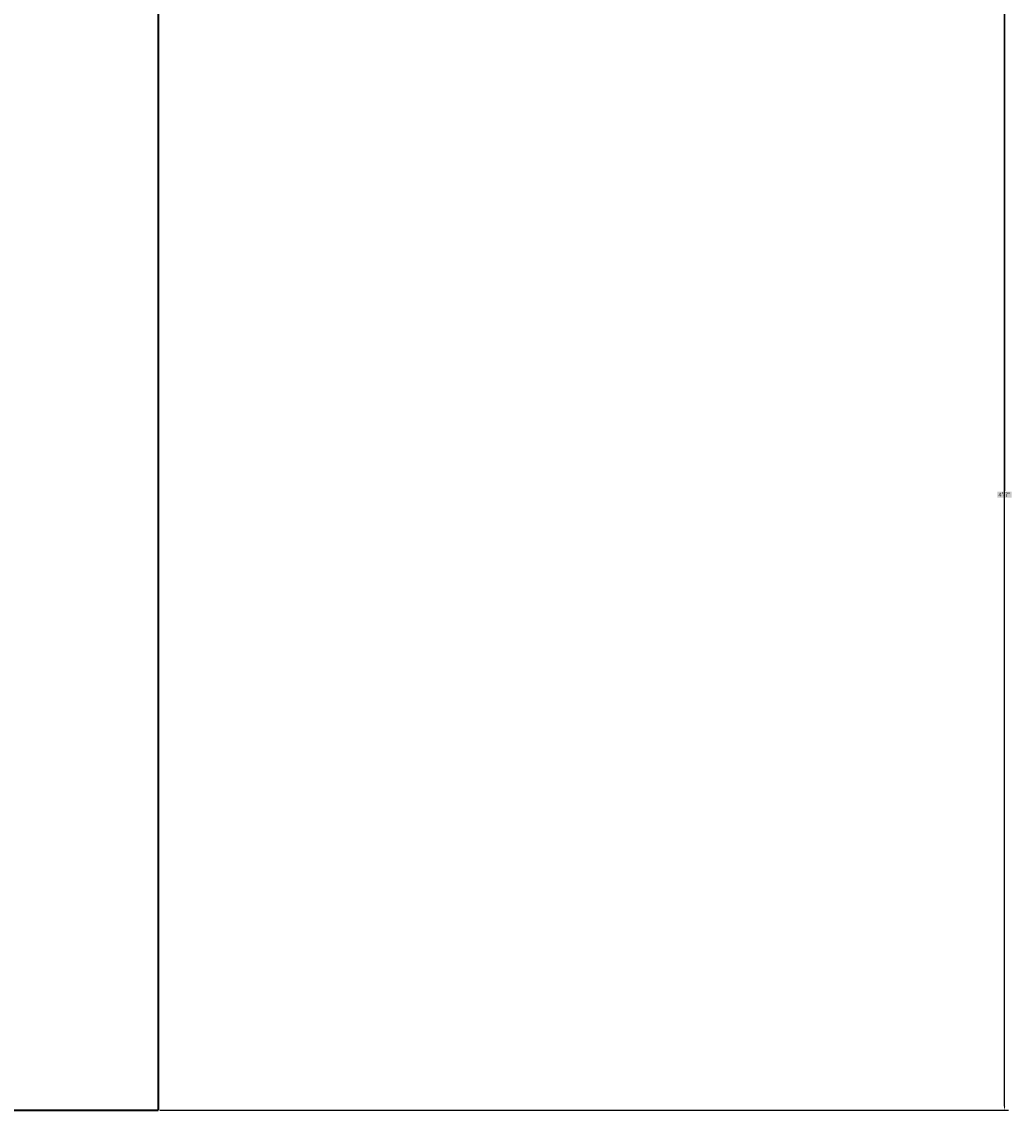
# Model space of a CAD drawing. Units: inches. Extents: x -128 to 854, y -395 to 398.
# Tile 28 of 61: x 308 to 352, y -89 to -41. Entities that reach past the tile are written whole.
import ezdxf

# ---------------------------------------------------------------- set-up
doc = ezdxf.new("R2010")
doc.units = ezdxf.units.IN
doc.header["$MEASUREMENT"] = 0
doc.layers.add('A-ANNO-DIMS', color=2, linetype='Continuous', lineweight=18)
doc.layers.add('A-WALL', color=4, linetype='Continuous', lineweight=35)
doc.styles.get("Standard").update_dxf_attribs({"font": 'arial.ttf'})
doc.dimstyles.get("Standard").update_dxf_attribs({"dimtxt": 0.18, "dimasz": 0.18, "dimexe": 0.18, "dimexo": 0.0625, "dimgap": 0.09, "dimtad": 0, "dimtih": 1, "dimtoh": 1, "dimdec": 1, "dimzin": 0, "dimdsep": 46, "dimlunit": 4, "dimtxsty": 'Standard', "dimcen": 0.09, "dimclrd": 1, "dimclre": 2, "dimclrt": 6, "dimadec": 0, "dimazin": 0, "dimtfac": 1, "dimtdec": 1, "dimtofl": 0, "dimtmove": 0, "dimatfit": 3, "dimfxl": 1, "dimtfill": 2, "dimtfillclr": 3, "dimtolj": 1, "dimtzin": 0, "dimarcsym": 0})

# ---------------------------------------------------------------- blocks, each defined once
blk = doc.blocks.new('*D98')
at = {"layer": 'A-ANNO-DIMS', "color": 2, "lineweight": -2, "transparency": 16777216}
for p, q in [((313.935, 348.741), (351.853, 348.741)), ((313.935, -89.259), (351.853, -89.259))]:
    blk.add_line(p, q, dxfattribs=at)
at = {"layer": 'A-ANNO-DIMS', "color": 1, "lineweight": -2, "transparency": 16777216}
for p, q in [((351.673, 348.561), (351.673, 129.923)), ((351.673, -89.079), (351.673, 129.559))]:
    blk.add_line(p, q, dxfattribs=at)
at = {"layer": 'A-ANNO-DIMS', "color": 1, "transparency": 16777216}
for points in [[(351.643, 348.561), (351.703, 348.561), (351.673, 348.741)], [(351.643, -89.079), (351.703, -89.079), (351.673, -89.259)]]:
    blk.add_solid(points, dxfattribs=at)
at = {"layer": 'Defpoints', "color": 0, "transparency": 16777216}
for p in [(313.873, 348.741), (351.673, 348.741), (313.873, -89.259)]:
    blk.add_point(p, dxfattribs=at)
at = {"layer": 'A-ANNO-DIMS', "color": 6, "transparency": 16777216, "insert": (351.673, 129.741), "char_height": 0.18, "attachment_point": 5, "bg_fill": 1, "box_fill_scale": 1.25, "bg_fill_color": 3, "bg_fill_transparency": 0}
blk.add_mtext('\\A1;36\'-6"', dxfattribs=at)
blk = doc.blocks.new('*D111')
at = {"layer": 'A-ANNO-DIMS', "color": 2, "lineweight": -2, "transparency": 16777216}
for p, q in [((313.935196, -34.259459), (351.852696, -34.259459)), ((313.935196, -89.259459), (351.852696, -89.259459))]:
    blk.add_line(p, q, dxfattribs=at)
at = {"layer": 'A-ANNO-DIMS', "color": 1, "lineweight": -2, "transparency": 16777216}
for p, q in [((351.672696, -34.439459), (351.672696, -61.579459)), ((351.672696, -89.079459), (351.672696, -61.939459))]:
    blk.add_line(p, q, dxfattribs=at)
at = {"layer": 'A-ANNO-DIMS', "color": 1, "transparency": 16777216}
for points in [[(351.642696, -34.439459), (351.702696, -34.439459), (351.672696, -34.259459)], [(351.642696, -89.079459), (351.702696, -89.079459), (351.672696, -89.259459)]]:
    blk.add_solid(points, dxfattribs=at)
at = {"layer": 'Defpoints', "color": 0, "transparency": 16777216}
for p in [(313.872696, -34.259459), (351.672696, -34.259459), (313.872696, -89.259459)]:
    blk.add_point(p, dxfattribs=at)
at = {"layer": 'A-ANNO-DIMS', "color": 6, "transparency": 16777216, "insert": (351.672696, -61.759459), "char_height": 0.18, "attachment_point": 5, "bg_fill": 1, "box_fill_scale": 1.25, "bg_fill_color": 3, "bg_fill_transparency": 0}
blk.add_mtext('\\A1;4\'-7"', dxfattribs=at)

msp = doc.modelspace()

# ---------------------------------------------------------------- linework, layer by layer
at = {"layer": 'A-WALL'}
for p in [(313.873, 348.741), (156.873, -89.259)]:
    msp.add_line(p, (313.873, -89.259), dxfattribs=at)

# ---------------------------------------------------------------- dimensions: what is measured, and where the dimension line sits
at = {"layer": 'A-ANNO-DIMS'}
for base, p2, picture, middle in [((351.673, 348.741), (313.873, 348.741), '*D98', (351.673, 129.741)), ((351.673, -34.259), (313.873, -34.259), '*D111', (351.673, -61.759))]:
    dim = msp.add_linear_dim(base=base, p1=(313.873, -89.259), p2=p2, angle=90, dimstyle='Standard', override={"dimdec": 1, "dimlfac": 1, "dimrnd": 0, "dimzin": 1, "dimdsep": 46, "dimlunit": 4, "dimfrac": 2}, dxfattribs=at)
    dim.commit()
    dim.dimension.update_dxf_attribs({"geometry": picture, "text_midpoint": middle})

doc.saveas('drawing.dxf')
